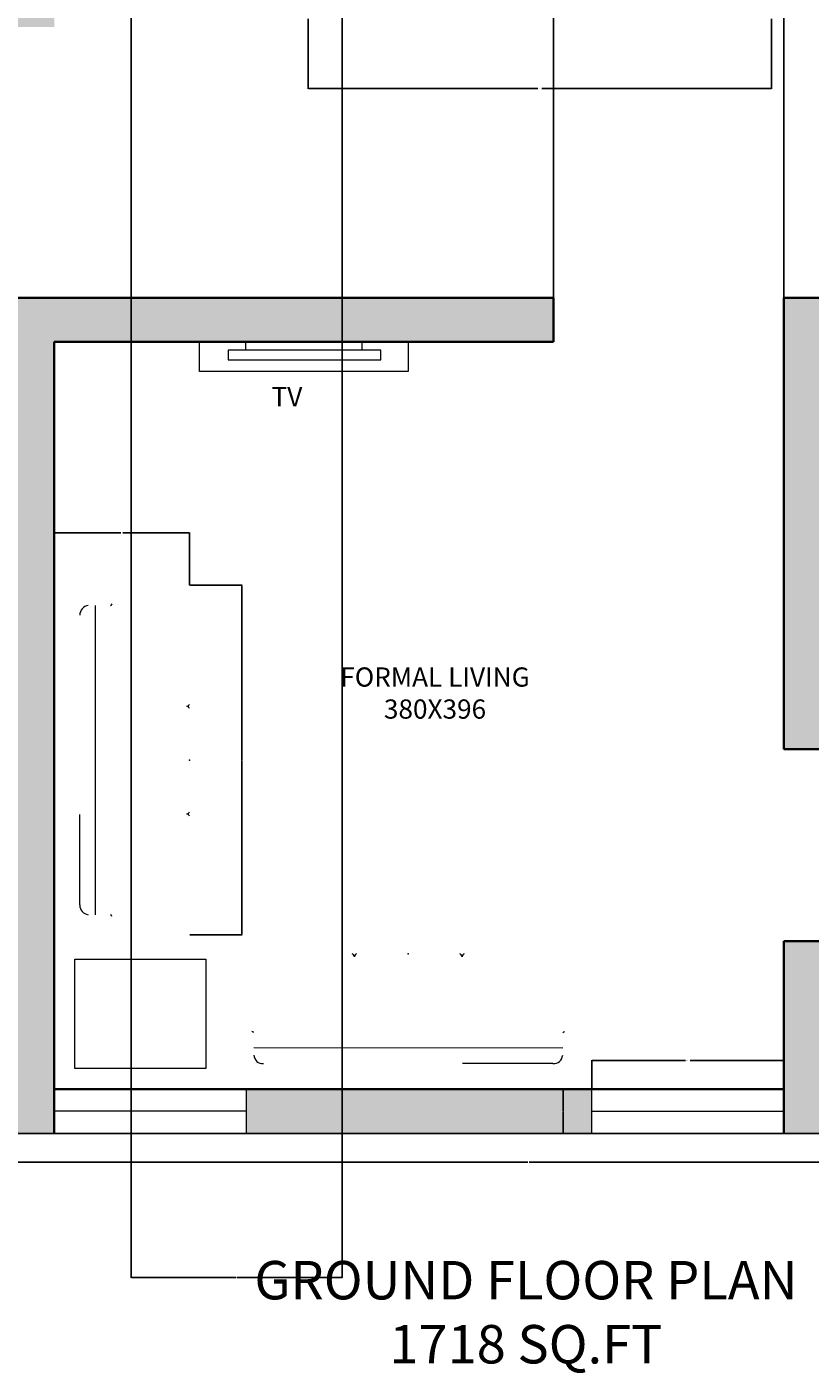
# Model space of a CAD drawing. Units: centimetres. Extents: x 2178 to 3635, y 1064 to 2635.
# Tile 3 of 9: x 2645 to 3053, y 1064 to 1765. Entities that reach past the tile are written whole.
import ezdxf

# ---------------------------------------------------------------- set-up
doc = ezdxf.new("R2010")
doc.units = ezdxf.units.CM
for name, color, linetype, lineweight in [('A-ANNO-DIMS', 2, 'Continuous', 18), ('A-ANNO-TEXT', 7, 'Continuous', 18), ('A-AREA-IDEN', 7, 'Continuous', 18), ('A-EQPM', 42, 'Continuous', 18), ('A-FLOR', 7, 'Continuous', 25), ('A-FURN', 42, 'Continuous', 18), ('A-GLAZ', 4, 'Continuous', 18), ('A-WALL', 7, 'Continuous', 35)]:
    doc.layers.add(name, color=color, linetype=linetype, lineweight=lineweight)
doc.layers.add('A-WALL-PATT', color=18, linetype='Continuous', lineweight=13, true_color=0x000000)
doc.styles.get("Standard").update_dxf_attribs({"font": 'arial.ttf'})
doc.dimstyles.get("Standard").update_dxf_attribs({"dimtxt": 0.18, "dimasz": 0.18, "dimexe": 0.18, "dimexo": 0.0625, "dimgap": 0.09, "dimtad": 0, "dimtih": 1, "dimtoh": 1, "dimdec": 4, "dimzin": 0, "dimdsep": 46, "dimtxsty": 'Standard', "dimcen": 0.09, "dimadec": 0, "dimazin": 0, "dimtfac": 1, "dimtdec": 4, "dimtofl": 0, "dimtmove": 0, "dimatfit": 3, "dimfxl": 1, "dimtolj": 1, "dimtzin": 0, "dimarcsym": 0})

# ---------------------------------------------------------------- blocks, each defined once
blk = doc.blocks.new('Clinicians and patient chairs 9_dwgmodels.com')
at = {"color": 0}
for points in [[(-907.9, 0, 0, 0, 0), (-959.6, -11.1, 4.62, 4.62, 0)], [(907.9, 0, 0, 0, 0), (-907.9, 0, 4.62, 4.62, 0)], [(959.6, -11.1, 0, 0, 0), (907.9, 0, 4.62, 4.62, 0)], [(-1015.6, -68.3, 0, 0, 0), (-1025.5, -106.3, 4.62, 4.62, 0)], [(-994.7, -35.9, 0, 0, 0), (-1015.6, -68.3, 4.62, 4.62, 0)], [(-959.6, -11.1, 0, 0, 0), (-994.7, -35.9, 4.62, 4.62, 0)], [(994.7, -35.9, 0, 0, 0), (959.6, -11.1, 4.62, 4.62, 0)], [(1015.6, -68.3, 0, 0, 0), (994.7, -35.9, 4.62, 4.62, 0)], [(1025.5, -106.3, 0, 0, 0), (1015.6, -68.3, 4.62, 4.62, 0)], [(-1025.5, -106.3, 0, 0, 0), (-1025.5, -779.5, 4.62, 4.62, 0)], [(-313.4, -149.9, 0, 0, 0), (-318.1, -149.9, 4.62, 4.62, 0)], [(-314.5, -150.4, 0, 0, 0), (-315.7, -159.3, 4.62, 4.62, 0)], [(-315.7, -159.3, 0, 0, 0), (-315.7, -777.3, 4.62, 4.62, 0)], [(-309.5, -148.3, 0, 0, 0), (-314.5, -150.4, 4.62, 4.62, 0)], [(-308, -148.3, 0, 0, 0), (-309.5, -148.3, 4.62, 4.62, 0)], [(-307.5, -148.3, 0, 0, 0), (-308, -148.3, 4.62, 4.62, 0)], [(242.9, -148.3, 0, 0, 0), (-307.5, -148.3, 4.62, 4.62, 0)], [(242.9, -148.3, 0, 0, 0), (296, -148.3, 4.62, 4.62, 0)], [(296, -148.3, 0, 0, 0), (307.5, -148.3, 4.62, 4.62, 0)], [(308, -148.3, 0, 0, 0), (307.5, -148.3, 4.62, 4.62, 0)], [(309.5, -148.3, 0, 0, 0), (308, -148.3, 4.62, 4.62, 0)], [(309.5, -148.3, 0, 0, 0), (314.5, -150.4, 4.62, 4.62, 0)], [(849.5, -149.9, 0, 0, 0), (313.4, -149.9, 4.62, 4.62, 0)], [(314.5, -150.4, 0, 0, 0), (315.7, -159.3, 4.62, 4.62, 0)], [(315.7, -159.3, 0, 0, 0), (315.7, -777.3, 4.62, 4.62, 0)], [(1025.5, -779.5, 0, 0, 0), (1025.5, -106.3, 4.62, 4.62, 0)], [(1025.5, -779.5, 0, 0, 0), (1025.5, -117.3, 4.62, 4.62, 0)], [(-906.6, -285, 0, 0, 0), (-906.4, -198.1, 4.62, 4.62, 0)], [(315.7, -161.8, 0, 0, 0), (315.7, -777.3, 4.62, 4.62, 0)], [(906.9, -327, 0, 0, 0), (906.4, -199.7, 4.62, 4.62, 0)], [(-906.8, -305.4, 0, 0, 0), (-906.9, -324.5, 4.62, 4.62, 0)], [(-906.6, -285, 0, 0, 0), (-906.8, -305.4, 4.62, 4.62, 0)], [(-1023, -329.7, 0, 0, 0), (-1019.2, -332.9, 4.62, 4.62, 0)], [(-1019.8, -340.2, 0, 0, 0), (-1023, -348.6, 4.62, 4.62, 0)], [(-1010.3, -335.9, 0, 0, 0), (-1019.8, -340.2, 4.62, 4.62, 0)], [(-1019.2, -332.9, 0, 0, 0), (-1019, -333, 4.62, 4.62, 0)], [(-1019, -333, 0, 0, 0), (-1018.9, -333.1, 4.62, 4.62, 0)], [(-1013.9, -334.2, 0, 0, 0), (-1018.9, -333.1, 4.62, 4.62, 0)], [(-1013.9, -334.2, 0, 0, 0), (-964.4, -335.7, 4.62, 4.62, 0)], [(-917.1, -337, 0, 0, 0), (-1010.3, -335.9, 4.62, 4.62, 0)], [(-964.4, -335.7, 0, 0, 0), (-927.1, -336.8, 4.62, 4.62, 0)], [(-906.9, -324.5, 0, 0, 0), (-906.9, -329.8, 4.62, 4.62, 0)], [(906.9, -327, 0, 0, 0), (906.9, -329.9, 4.62, 4.62, 0)], [(964.4, -335.7, 0, 0, 0), (914.9, -337.2, 4.62, 4.62, 0)], [(917.1, -339.4, 0, 0, 0), (1010.3, -338.4, 4.62, 4.62, 0)], [(1013.9, -334.2, 0, 0, 0), (964.4, -335.7, 4.62, 4.62, 0)], [(1010.3, -338.4, 0, 0, 0), (1019.8, -342.7, 4.62, 4.62, 0)], [(1013.9, -334.2, 0, 0, 0), (1018.9, -333.1, 4.62, 4.62, 0)], [(1018.9, -333.1, 0, 0, 0), (1019, -333, 4.62, 4.62, 0)], [(1019.2, -332.9, 0, 0, 0), (1019, -333, 4.62, 4.62, 0)], [(1023, -329.7, 0, 0, 0), (1019.2, -332.9, 4.62, 4.62, 0)], [(1019.8, -342.7, 0, 0, 0), (1023, -351.1, 4.62, 4.62, 0)], [(1023, -351.1, 0, 0, 0), (1022.6, -779.8, 4.62, 4.62, 0)], [(-1025.5, -779.5, 0, 0, 0), (-1022.2, -788.7, 4.62, 4.62, 0)], [(-1022.2, -788.7, 0, 0, 0), (-1021.6, -789.8, 4.62, 4.62, 0)], [(-1021.6, -789.8, 0, 0, 0), (-1020.6, -790.5, 4.62, 4.62, 0)], [(-1020.6, -790.5, 0, 0, 0), (-1013.6, -793.7, 4.62, 4.62, 0)], [(1019.8, -788.8, 0, 0, 0), (1013.1, -793.7, 4.62, 4.62, 0)], [(1013.6, -793.7, 0, 0, 0), (1020.6, -790.5, 4.62, 4.62, 0)], [(1022.6, -779.8, 0, 0, 0), (1019.8, -788.8, 4.62, 4.62, 0)], [(1020.6, -790.5, 0, 0, 0), (1021.6, -789.8, 4.62, 4.62, 0)], [(1022.2, -788.7, 0, 0, 0), (1021.6, -789.8, 4.62, 4.62, 0)], [(1022.2, -788.7, 0, 0, 0), (1025.5, -779.5, 4.62, 4.62, 0)], [(-1013.6, -793.7, 0, 0, 0), (1013.6, -793.7, 4.62, 4.62, 0)]]:
    blk.add_lwpolyline(points, format="xyseb", dxfattribs=at)
for points in [[(-849.5, -149.9), (-318.1, -149.9)], [(-906.5, -241.5), (906.5, -242.3)]]:
    blk.add_lwpolyline(points, dxfattribs=at)
for centre, radius, start, end in [((-851.7, -204.8), 54.9, 87.66794, 174.72556), ((851.7, -204.8), 54.9, 5.27444, 92.33206), ((-916.6, -326.8), 10.2, 267.54544, 342.40568), ((916.9, -329.4), 10, 182.60942, 270.79497), ((-337, -773.8), 21.5, 292.11503, 350.63044), ((-294.5, -773.8), 21.5, 189.36956, 247.88497), ((294.5, -773.8), 21.5, 292.11503, 350.63044), ((336.9, -773.8), 21.5, 189.36956, 247.88497)]:
    blk.add_arc(centre, radius, start, end, dxfattribs=at)
blk.add_point((0, -793.7), dxfattribs=at)
blk = doc.blocks.new('WIN-1000')
for p, q in [((100, 23), (100, 0)), ((100, 11.5), (0, 11.5))]:
    blk.add_line(p, q)
blk = doc.blocks.new('*D34')
at = {"layer": 'A-ANNO-DIMS', "color": 0, "lineweight": -2, "transparency": 16777216}
for p, q in [((2730.13, 1473.95), (2757.56, 1473.95)), ((2757.38, 1473.77), (2757.38, 1383.1)), ((2757.38, 1292.06), (2757.38, 1382.73)), ((2730.13, 1291.88), (2757.56, 1291.88))]:
    blk.add_line(p, q, dxfattribs=at)
at = {"layer": 'A-ANNO-DIMS', "color": 0, "transparency": 16777216}
for points in [[(2757.35, 1473.77), (2757.41, 1473.77), (2757.38, 1473.95)], [(2757.35, 1292.06), (2757.41, 1292.06), (2757.38, 1291.88)]]:
    blk.add_solid(points, dxfattribs=at)
at = {"layer": 'Defpoints', "color": 0, "transparency": 16777216}
for p in [(2730.07, 1473.95), (2757.38, 1473.95), (2730.07, 1291.88)]:
    blk.add_point(p, dxfattribs=at)
at = {"layer": 'A-ANNO-DIMS', "color": 0, "transparency": 16777216, "insert": (2757.38, 1382.92), "char_height": 0.18, "attachment_point": 5}
blk.add_mtext('\\A1;SOFA 182 TYP.', dxfattribs=at)
blk = doc.blocks.new('*D35')
at = {"layer": 'A-ANNO-DIMS', "color": 0, "lineweight": -2, "transparency": 16777216}
for p, q in [((2659.6, 1474.02), (2659.6, 1501.45)), ((2659.78, 1501.27), (2694.31, 1501.27)), ((2729.89, 1501.27), (2695.36, 1501.27)), ((2730.07, 1474.02), (2730.07, 1501.45))]:
    blk.add_line(p, q, dxfattribs=at)
at = {"layer": 'A-ANNO-DIMS', "color": 0, "transparency": 16777216}
for points in [[(2659.78, 1501.3), (2659.78, 1501.24), (2659.6, 1501.27)], [(2729.89, 1501.3), (2729.89, 1501.24), (2730.07, 1501.27)]]:
    blk.add_solid(points, dxfattribs=at)
at = {"layer": 'Defpoints', "color": 0, "transparency": 16777216}
for p in [(2659.6, 1501.27), (2659.6, 1473.95), (2730.07, 1473.95)]:
    blk.add_point(p, dxfattribs=at)
at = {"layer": 'A-ANNO-DIMS', "color": 0, "transparency": 16777216, "insert": (2694.84, 1501.27), "char_height": 0.18, "attachment_point": 5}
blk.add_mtext('\\A1;70 TYP.', dxfattribs=at)
blk = doc.blocks.new('*D36')
at = {"layer": 'A-ANNO-DIMS', "color": 0, "lineweight": -2, "transparency": 16777216}
for p, q in [((2939.6, 1211.65), (2939.6, 1226.77)), ((2939.78, 1226.59), (2988.42, 1226.59)), ((3039.42, 1226.59), (2990.79, 1226.59)), ((3039.6, 1211.65), (3039.6, 1226.77))]:
    blk.add_line(p, q, dxfattribs=at)
at = {"layer": 'A-ANNO-DIMS', "color": 0, "transparency": 16777216}
for points in [[(2939.78, 1226.62), (2939.78, 1226.56), (2939.6, 1226.59)], [(3039.42, 1226.62), (3039.42, 1226.56), (3039.6, 1226.59)]]:
    blk.add_solid(points, dxfattribs=at)
at = {"layer": 'Defpoints', "color": 0, "transparency": 16777216}
for p in [(2939.6, 1226.59), (2939.6, 1211.59), (3039.6, 1211.59)]:
    blk.add_point(p, dxfattribs=at)
at = {"layer": 'A-ANNO-DIMS', "color": 0, "transparency": 16777216, "insert": (2989.6, 1226.59), "char_height": 0.18, "attachment_point": 5}
blk.add_mtext('\\A1;WINDOW 100 TYP.', dxfattribs=at)
blk = doc.blocks.new('*D37')
at = {"layer": 'A-ANNO-DIMS', "color": 0, "lineweight": -2, "transparency": 16777216}
for p, q in [((2939.54, 1211.59), (2924.42, 1211.59)), ((2924.6, 1211.41), (2924.6, 1200.27)), ((2924.6, 1188.77), (2924.6, 1199.91)), ((2939.54, 1188.59), (2924.42, 1188.59))]:
    blk.add_line(p, q, dxfattribs=at)
at = {"layer": 'A-ANNO-DIMS', "color": 0, "transparency": 16777216}
for points in [[(2924.57, 1211.41), (2924.63, 1211.41), (2924.6, 1211.59)], [(2924.57, 1188.77), (2924.63, 1188.77), (2924.6, 1188.59)]]:
    blk.add_solid(points, dxfattribs=at)
at = {"layer": 'Defpoints', "color": 0, "transparency": 16777216}
for p in [(2939.6, 1211.59), (2924.6, 1188.59), (2939.6, 1188.59)]:
    blk.add_point(p, dxfattribs=at)
at = {"layer": 'A-ANNO-DIMS', "color": 0, "transparency": 16777216, "insert": (2924.6, 1200.09), "char_height": 0.18, "attachment_point": 5}
blk.add_mtext('\\A1;23 TYP.', dxfattribs=at)
blk = doc.blocks.new('*D40')
at = {"layer": 'A-ANNO-DIMS', "color": 0, "lineweight": -2, "transparency": 16777216}
for p, q in [((2791.91, 1768.73), (2791.91, 1732.42)), ((3033.17, 1768.73), (3033.17, 1732.42)), ((2792.09, 1732.6), (2911.51, 1732.6)), ((3032.99, 1732.6), (2913.56, 1732.6))]:
    blk.add_line(p, q, dxfattribs=at)
at = {"layer": 'A-ANNO-DIMS', "color": 0, "transparency": 16777216}
for points in [[(2792.09, 1732.63), (2792.09, 1732.57), (2791.91, 1732.6)], [(3032.99, 1732.63), (3032.99, 1732.57), (3033.17, 1732.6)]]:
    blk.add_solid(points, dxfattribs=at)
at = {"layer": 'Defpoints', "color": 0, "transparency": 16777216}
for p in [(2791.91, 1768.79), (3033.17, 1768.79), (3033.17, 1732.6)]:
    blk.add_point(p, dxfattribs=at)
at = {"layer": 'A-ANNO-DIMS', "color": 0, "transparency": 16777216, "insert": (2912.54, 1732.6), "char_height": 0.18, "attachment_point": 5}
blk.add_mtext('\\A1;DINING SET 241', dxfattribs=at)
blk = doc.blocks.new('*D46')
at = {"layer": 'A-ANNO-DIMS', "color": 0, "lineweight": -2, "transparency": 16777216}
for p, q in [((2253.6, 1248.53), (2253.6, 1173.41)), ((3559.6, 1248.53), (3559.6, 1173.41)), ((2253.78, 1173.59), (2906.25, 1173.59)), ((3559.42, 1173.59), (2906.95, 1173.59))]:
    blk.add_line(p, q, dxfattribs=at)
at = {"layer": 'A-ANNO-DIMS', "color": 0, "transparency": 16777216}
for points in [[(2253.78, 1173.62), (2253.78, 1173.56), (2253.6, 1173.59)], [(3559.42, 1173.62), (3559.42, 1173.56), (3559.6, 1173.59)]]:
    blk.add_solid(points, dxfattribs=at)
at = {"layer": 'Defpoints', "color": 0, "transparency": 16777216}
for p in [(2253.6, 1248.59), (3559.6, 1248.59), (2253.6, 1173.59)]:
    blk.add_point(p, dxfattribs=at)
at = {"layer": 'A-ANNO-DIMS', "color": 0, "transparency": 16777216, "insert": (2906.6, 1173.59), "char_height": 0.18, "attachment_point": 5}
blk.add_mtext('\\A1;1306', dxfattribs=at)
blk = doc.blocks.new('*D61')
at = {"layer": 'A-ANNO-DIMS', "color": 0, "lineweight": -2, "transparency": 16777216}
for p, q in [((2919.6, 1623.65), (2919.6, 2634.77)), ((2919.78, 2634.59), (2979.32, 2634.59)), ((3039.42, 2634.59), (2979.88, 2634.59)), ((3039.6, 1623.65), (3039.6, 2634.77))]:
    blk.add_line(p, q, dxfattribs=at)
at = {"layer": 'A-ANNO-DIMS', "color": 0, "transparency": 16777216}
for points in [[(2919.78, 2634.62), (2919.78, 2634.56), (2919.6, 2634.59)], [(3039.42, 2634.62), (3039.42, 2634.56), (3039.6, 2634.59)]]:
    blk.add_solid(points, dxfattribs=at)
at = {"layer": 'Defpoints', "color": 0, "transparency": 16777216}
for p in [(3039.6, 2634.59), (2919.6, 1623.59), (3039.6, 1623.59)]:
    blk.add_point(p, dxfattribs=at)
at = {"layer": 'A-ANNO-DIMS', "color": 0, "transparency": 16777216, "insert": (2979.6, 2634.59), "char_height": 0.18, "attachment_point": 5}
blk.add_mtext('\\A1;120', dxfattribs=at)
blk = doc.blocks.new('*D63')
at = {"layer": 'A-ANNO-DIMS', "color": 0, "lineweight": -2, "transparency": 16777216}
for p, q in [((2699.6, 2093.53), (2699.6, 1113.41)), ((2809.6, 2093.53), (2809.6, 1113.41)), ((2699.78, 1113.59), (2754.32, 1113.59)), ((2809.42, 1113.59), (2754.88, 1113.59))]:
    blk.add_line(p, q, dxfattribs=at)
at = {"layer": 'A-ANNO-DIMS', "color": 0, "transparency": 16777216}
for points in [[(2699.78, 1113.62), (2699.78, 1113.56), (2699.6, 1113.59)], [(2809.42, 1113.62), (2809.42, 1113.56), (2809.6, 1113.59)]]:
    blk.add_solid(points, dxfattribs=at)
at = {"layer": 'Defpoints', "color": 0, "transparency": 16777216}
for p in [(2699.6, 2093.59), (2809.6, 2093.59), (2809.6, 1113.59)]:
    blk.add_point(p, dxfattribs=at)
at = {"layer": 'A-ANNO-DIMS', "color": 0, "transparency": 16777216, "insert": (2754.6, 1113.59), "char_height": 0.18, "attachment_point": 5}
blk.add_mtext('\\A1;110', dxfattribs=at)
blk = doc.blocks.new('*D78')
at = {"layer": 'A-ANNO-DIMS', "color": 0, "lineweight": -2, "transparency": 16777216}
for p, q in [((3039.67, 1388.59), (3114.78, 1388.59)), ((3114.6, 1388.41), (3114.6, 1338.77)), ((3114.6, 1288.77), (3114.6, 1338.41)), ((3039.67, 1288.59), (3114.78, 1288.59))]:
    blk.add_line(p, q, dxfattribs=at)
at = {"layer": 'A-ANNO-DIMS', "color": 0, "transparency": 16777216}
for points in [[(3114.57, 1388.41), (3114.63, 1388.41), (3114.6, 1388.59)], [(3114.57, 1288.77), (3114.63, 1288.77), (3114.6, 1288.59)]]:
    blk.add_solid(points, dxfattribs=at)
at = {"layer": 'Defpoints', "color": 0, "transparency": 16777216}
for p in [(3039.6, 1388.59), (3039.6, 1288.59), (3114.6, 1288.59)]:
    blk.add_point(p, dxfattribs=at)
at = {"layer": 'A-ANNO-DIMS', "color": 0, "transparency": 16777216, "insert": (3114.6, 1338.59), "char_height": 0.18, "attachment_point": 5}
blk.add_mtext('\\A1;100', dxfattribs=at)

msp = doc.modelspace()

# ---------------------------------------------------------------- hatches: boundary and pattern name
at = {"layer": 'A-WALL-PATT'}
h = msp.add_hatch(color=256, dxfattribs=at)
h.dxf.hatch_style = 1
h.paths.add_polyline_path([(2276.605, 2499.59), (2253.605, 2499.59), (2253.605, 2476.59), (2276.605, 2476.59)])
h.paths.add_polyline_path([(2411.605, 2350.59), (2253.605, 2350.59), (2253.605, 2327.59), (2411.605, 2327.59)])
h.paths.add_polyline_path([(2276.605, 2252.59), (2253.605, 2252.59), (2253.605, 2020.59), (2276.605, 2020.59), (2276.605, 2093.59), (2561.605, 2093.59), (2561.605, 2116.59), (2276.605, 2116.59)])
h.paths.add_polyline_path([(2659.605, 1787.59), (2610.616, 1787.59), (2276.605, 1787.59), (2276.605, 1860.59), (2253.605, 1860.59), (2253.605, 1732.09), (2276.605, 1732.09), (2276.605, 1764.59), (2516.605, 1764.59), (2516.605, 1699.59), (2539.605, 1699.59), (2539.605, 1764.59), (2659.605, 1764.59)])
h.paths.add_polyline_path([(2539.605, 1624.59), (2276.605, 1624.59), (2276.605, 1657.09), (2253.605, 1657.09), (2253.605, 1561.59), (2276.605, 1561.59), (2276.605, 1601.59), (2539.605, 1601.59)])
h.paths.add_polyline_path([(2276.605, 1501.59), (2253.605, 1501.59), (2253.605, 1371.59), (2276.605, 1371.59)])
h.paths.add_polyline_path([(2376.605, 1271.59), (2276.605, 1271.59), (2276.605, 1311.59), (2253.605, 1311.59), (2253.605, 1248.59), (2376.605, 1248.59)])
h.paths.add_polyline_path([(2636.605, 1271.59), (2536.605, 1271.59), (2536.605, 1248.59), (2636.605, 1248.59)])
h.paths.add_polyline_path([(2659.605, 1600.59), (2919.605, 1600.59), (2919.605, 1623.59), (2636.605, 1623.59), (2636.605, 1188.59), (2659.605, 1188.59)])
h.paths.add_polyline_path([(2939.605, 1211.59), (2759.605, 1211.59), (2759.605, 1188.59), (2939.605, 1188.59)])
h.paths.add_polyline_path([(3062.605, 1288.59), (3039.605, 1288.59), (3039.605, 1188.59), (3062.605, 1188.59)])
h.paths.add_polyline_path([(3372.605, 1248.59), (3062.605, 1248.59), (3062.605, 1218.59), (3372.605, 1218.59)])
h.paths.add_polyline_path([(3395.605, 1271.59), (3372.605, 1271.59), (3372.605, 1248.59), (3395.605, 1248.59)])
h.paths.add_polyline_path([(3559.605, 1271.59), (3536.605, 1271.59), (3536.605, 1248.59), (3559.605, 1248.59)])
h.paths.add_polyline_path([(3559.605, 1623.59), (3536.605, 1623.59), (3536.605, 1600.59), (3559.605, 1600.59)])
h.paths.add_polyline_path([(3395.605, 1623.59), (3162.605, 1623.59), (3162.605, 1600.59), (3395.605, 1600.59)])
h.paths.add_polyline_path([(3395.605, 1411.59), (3277.1, 1411.59), (3277.1, 1388.59), (3395.605, 1388.59)])
h.paths.add_polyline_path([(3157.1, 1411.59), (3062.605, 1411.59), (3062.605, 1623.59), (3039.605, 1623.59), (3039.605, 1388.59), (3157.1, 1388.59)])
h.paths.add_polyline_path([(3559.605, 1797.09), (3536.605, 1797.09), (3536.605, 1764.59), (3316.605, 1764.59), (3316.605, 1927.59), (3293.605, 1927.59), (3293.605, 1741.59), (3372.605, 1741.59), (3395.605, 1741.59), (3559.605, 1741.59)])
h.paths.add_polyline_path([(3559.605, 1990.59), (3536.605, 1990.59), (3536.605, 1974.446), (3536.605, 1927.59), (3391.605, 1927.59), (3391.605, 1904.59), (3536.605, 1904.59), (3536.605, 1872.09), (3559.605, 1872.09)])
h.paths.add_polyline_path([(3559.605, 2180.59), (3536.605, 2180.59), (3536.605, 2050.59), (3559.605, 2050.59)])
h.paths.add_polyline_path([(3559.605, 2326.59), (3446.105, 2326.59), (3446.105, 2303.59), (3536.605, 2303.59), (3536.605, 2240.59), (3559.605, 2240.59)])
h.paths.add_polyline_path([(3286.105, 2326.59), (3195.605, 2326.59), (3195.605, 2499.59), (3082.605, 2499.59), (3082.605, 2476.59), (3172.605, 2476.59), (3172.605, 2116.59), (2809.605, 2116.59), (2809.605, 2093.59), (3172.605, 2093.59), (3172.605, 1904.59), (3195.605, 1904.59), (3195.605, 2303.59), (3286.105, 2303.59)])
h.paths.add_polyline_path([(2832.605, 2236.59), (2659.605, 2236.59), (2659.605, 2476.59), (2697.105, 2476.59), (2697.105, 2499.59), (2636.605, 2499.59), (2636.605, 2093.59), (2699.605, 2093.59), (2699.605, 2116.59), (2659.605, 2116.59), (2659.605, 2213.59), (2832.605, 2213.59)])
h.paths.add_polyline_path([(2832.605, 2476.59), (2922.605, 2476.59), (2922.605, 2499.59), (2772.105, 2499.59), (2772.105, 2476.59), (2809.605, 2476.59), (2809.605, 2311.59), (2832.605, 2311.59)])

# ---------------------------------------------------------------- linework, layer by layer
at = {"layer": 'A-EQPM'}
for points in [[(2759.352, 1600.59), (2819.858, 1600.59), (2819.858, 1596.373), (2759.352, 1596.373)], [(2829.759, 1596.373), (2750.138, 1596.373), (2750.138, 1591.289), (2829.759, 1591.289)]]:
    msp.add_lwpolyline(points, close=True, dxfattribs=at)
at = {"layer": 'A-FLOR'}
msp.add_line((2253.605, 1188.59), (3559.605, 1188.59), dxfattribs=at)
at = {"layer": 'A-FURN'}
for points in [[(2735.301, 1600.59), (2843.908, 1600.59), (2843.908, 1585.212), (2735.301, 1585.212)], [(2670.363, 1279.293), (2738.466, 1279.293), (2738.466, 1222.298), (2670.363, 1222.298)]]:
    msp.add_lwpolyline(points, close=True, dxfattribs=at)
at = {"layer": 'A-WALL'}
for p, q in [((2636.605, 1623.59), (2919.605, 1623.59)), ((2919.605, 1623.59), (2919.605, 1600.59)), ((3039.605, 1623.59), (3039.605, 1388.59)), ((3039.605, 1623.59), (3062.605, 1623.59)), ((2659.605, 1600.59), (2919.605, 1600.59)), ((2659.605, 1600.59), (2659.605, 1188.59)), ((3039.605, 1388.59), (3395.605, 1388.59)), ((3039.605, 1288.59), (3062.605, 1288.59)), ((3039.605, 1288.59), (3039.605, 1188.59)), ((2659.605, 1211.59), (3039.605, 1211.59))]:
    msp.add_line(p, q, dxfattribs=at)

# ---------------------------------------------------------------- block references
at = {"layer": 'A-FURN', "xscale": 0.0887725350099512, "yscale": 0.0887725350099512, "zscale": 0.0887725350099512}
for p, rotation in [((2659.605, 1382.916), 89.99999999999999), ((2843.955, 1211.59), 180)]:
    msp.add_blockref('Clinicians and patient chairs 9_dwgmodels.com', p, dxfattribs=dict(at, rotation=rotation))
at = {"layer": 'A-GLAZ'}
msp.add_blockref('WIN-1000', (2659.605, 1188.59), dxfattribs=at)
at = {"layer": 'A-GLAZ', "rotation": 180}
msp.add_blockref('WIN-1000', (3039.605, 1211.59), dxfattribs=at)

# ---------------------------------------------------------------- texts
at = {"layer": 'A-ANNO-TEXT', "attachment_point": 1}
for s, width, insert, char_height in [('\\pxqc;TV', 111.5542, (2725.004, 1577.087), 10), ('\\pxqc;{\\fArial|b1|i1|c0|p34;GROUND FLOOR PLAN\\P1718 SQ.FT}', 512.84793, (2648.866, 1122.183), 20)]:
    msp.add_mtext_dynamic_manual_height_columns(s, width=width, gutter_width=12.5, heights=[0], dxfattribs=dict(at, insert=insert, char_height=char_height))
at = {"layer": 'A-AREA-IDEN', "insert": (2802.148, 1431.162), "char_height": 10, "attachment_point": 1}
msp.add_mtext_dynamic_manual_height_columns('\\pxqc;FORMAL LIVING\\P380X396', width=111.5542, gutter_width=12.5, heights=[0], dxfattribs=at)

# ---------------------------------------------------------------- dimensions: what is measured, and where the dimension line sits
at = {"layer": 'A-ANNO-DIMS'}
for base, p1, p2, picture, middle in [((3039.605, 2634.59), (2919.605, 1623.59), (3039.605, 1623.59), '*D61', (2979.605, 2634.59)), ((2809.605, 1113.59), (2699.605, 2093.59), (2809.605, 2093.59), '*D63', (2754.605, 1113.59))]:
    dim = msp.add_linear_dim(base=base, p1=p1, p2=p2, dimstyle='Standard', override={"dimdec": 0, "dimlfac": 1, "dimrnd": 0, "dimzin": 0, "dimdsep": 46, "dimlunit": 2}, dxfattribs=at)
    dim.commit()
    dim.dimension.update_dxf_attribs({"geometry": picture, "text_midpoint": middle})
dim = msp.add_linear_dim(base=(3033.166, 1732.601), p1=(2791.905, 1768.791), p2=(3033.166, 1768.791), text='DINING SET <>', dimstyle='Standard', override={"dimdec": 0, "dimlfac": 1, "dimrnd": 0, "dimzin": 0, "dimdsep": 46, "dimlunit": 2}, dxfattribs=at)
dim.commit()
dim.dimension.update_dxf_attribs({"geometry": '*D40', "text_midpoint": (2912.536, 1732.601)})
for base, p1, p2, angle, text, picture, middle in [((2659.605, 1501.265), (2730.067, 1473.954), (2659.605, 1473.954), 180, '<> TYP.', '*D35', (2694.836, 1501.265)), ((2757.378, 1473.954), (2730.067, 1291.878), (2730.067, 1473.954), 90, 'SOFA <> TYP.', '*D34', (2757.378, 1382.916)), ((2939.605, 1226.59), (3039.605, 1211.59), (2939.605, 1211.59), 180, 'WINDOW <> TYP.', '*D36', (2989.605, 1226.59)), ((2924.605, 1188.59), (2939.605, 1211.59), (2939.605, 1188.59), 270, '<> TYP.', '*D37', (2924.605, 1200.09))]:
    dim = msp.add_linear_dim(base=base, p1=p1, p2=p2, angle=angle, text=text, dimstyle='Standard', override={"dimdec": 0, "dimlfac": 1, "dimrnd": 0, "dimzin": 0, "dimdsep": 46, "dimlunit": 2}, dxfattribs=at)
    dim.commit()
    dim.dimension.update_dxf_attribs({"geometry": picture, "text_midpoint": middle})
for base, p1, p2, angle, picture, middle in [((3114.605, 1288.59), (3039.605, 1388.59), (3039.605, 1288.59), 270, '*D78', (3114.605, 1338.59)), ((2253.605, 1173.59), (3559.605, 1248.59), (2253.605, 1248.59), 180, '*D46', (2906.605, 1173.59))]:
    dim = msp.add_linear_dim(base=base, p1=p1, p2=p2, angle=angle, dimstyle='Standard', override={"dimdec": 0, "dimlfac": 1, "dimrnd": 0, "dimzin": 0, "dimdsep": 46, "dimlunit": 2}, dxfattribs=at)
    dim.commit()
    dim.dimension.update_dxf_attribs({"geometry": picture, "text_midpoint": middle})

doc.saveas('drawing.dxf')
